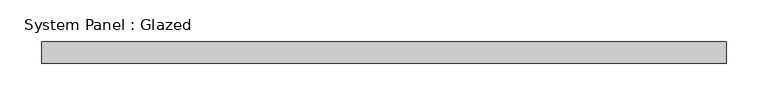
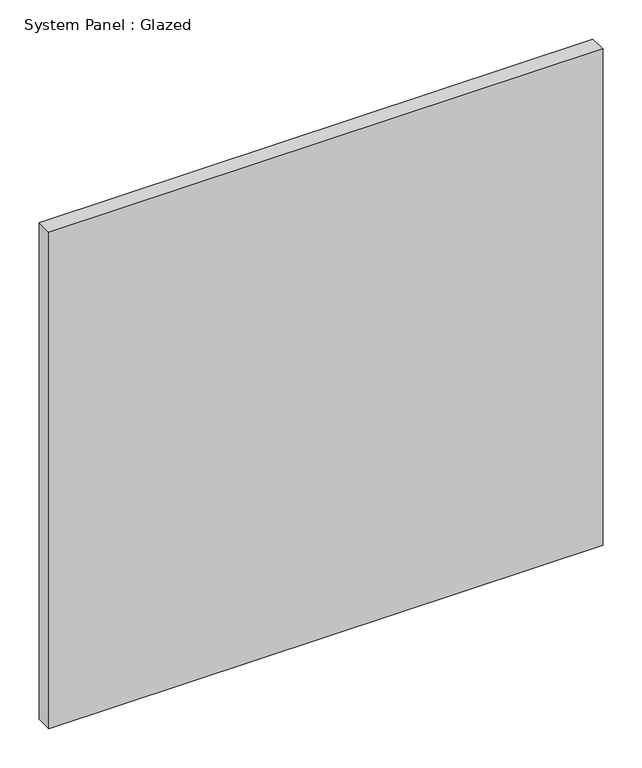
"""IFC4 building model written with IfcOpenShell, lengths in millimetres: plate geometry, System Panel : Glazed."""

from ifc_helpers import new_model, si_unit, origin, origin_with_axes, place, context, project, spatial, polyline, outline, extrude, source, transform, mapped, element, save


def system_panel_glazed_c1c9c451(model_context):
    return source(origin(), model_context, "Body", "SweptSolid", [
        extrude(outline(polyline([(409.575, 19.05), (-409.575, 19.05), (-409.575, 44.45), (409.575, 44.45), (409.575, 19.05)])), origin_with_axes(), (0.0, 0.0, 1.0), 776.0351947),
    ])


if __name__ == "__main__":
    model = new_model("IFC4")
    model_context = context("Model", 3, world=origin())
    ifc_project = project(units=[si_unit("LENGTHUNIT", "METRE", prefix="MILLI")], contexts=[model_context])
    site = spatial("IfcSite", under=ifc_project)
    building = spatial("IfcBuilding", under=site)
    placement = place(None, origin())
    system_panel_glazed_shape = system_panel_glazed_c1c9c451(model_context)
    element("IfcPlate", 1, ObjectType="System Panel : Glazed", at=placement, inside=building, context=model_context, shape_type="MappedRepresentation", body=[
        mapped(system_panel_glazed_shape, transform((0.0, 0.0, 0.0), x_axis=(1.0, 0.0, 0.0), y_axis=(0.0, 1.0, 0.0), z_axis=(0.0, 0.0, 1.0))),
    ])
    save(model, "model.ifc")

# Revit data of these elements
# Type "System Panel : Glazed"
#   Construction Type Id = "GSP4R"
#   Analytic Construction = "1/8 in Pilkington single glazing"
#   Visual Light Transmittance = 0.9
#   Solar Heat Gain Coefficient = 0.86
#   Heat Transfer Coefficient (U) = 1.18115 BTU/(h·ft²·°F)
#   Define Thermal Properties by = 1
# Element 1 (IfcPlate, "System Panel : Glazed")
#   Materials on its faces: "Glass"
# Materials
#   "Glass": class "Glass", colour RGB 0 128 192, transparency 0.75, Description = "Soda Lime Glass", Cost = 0
